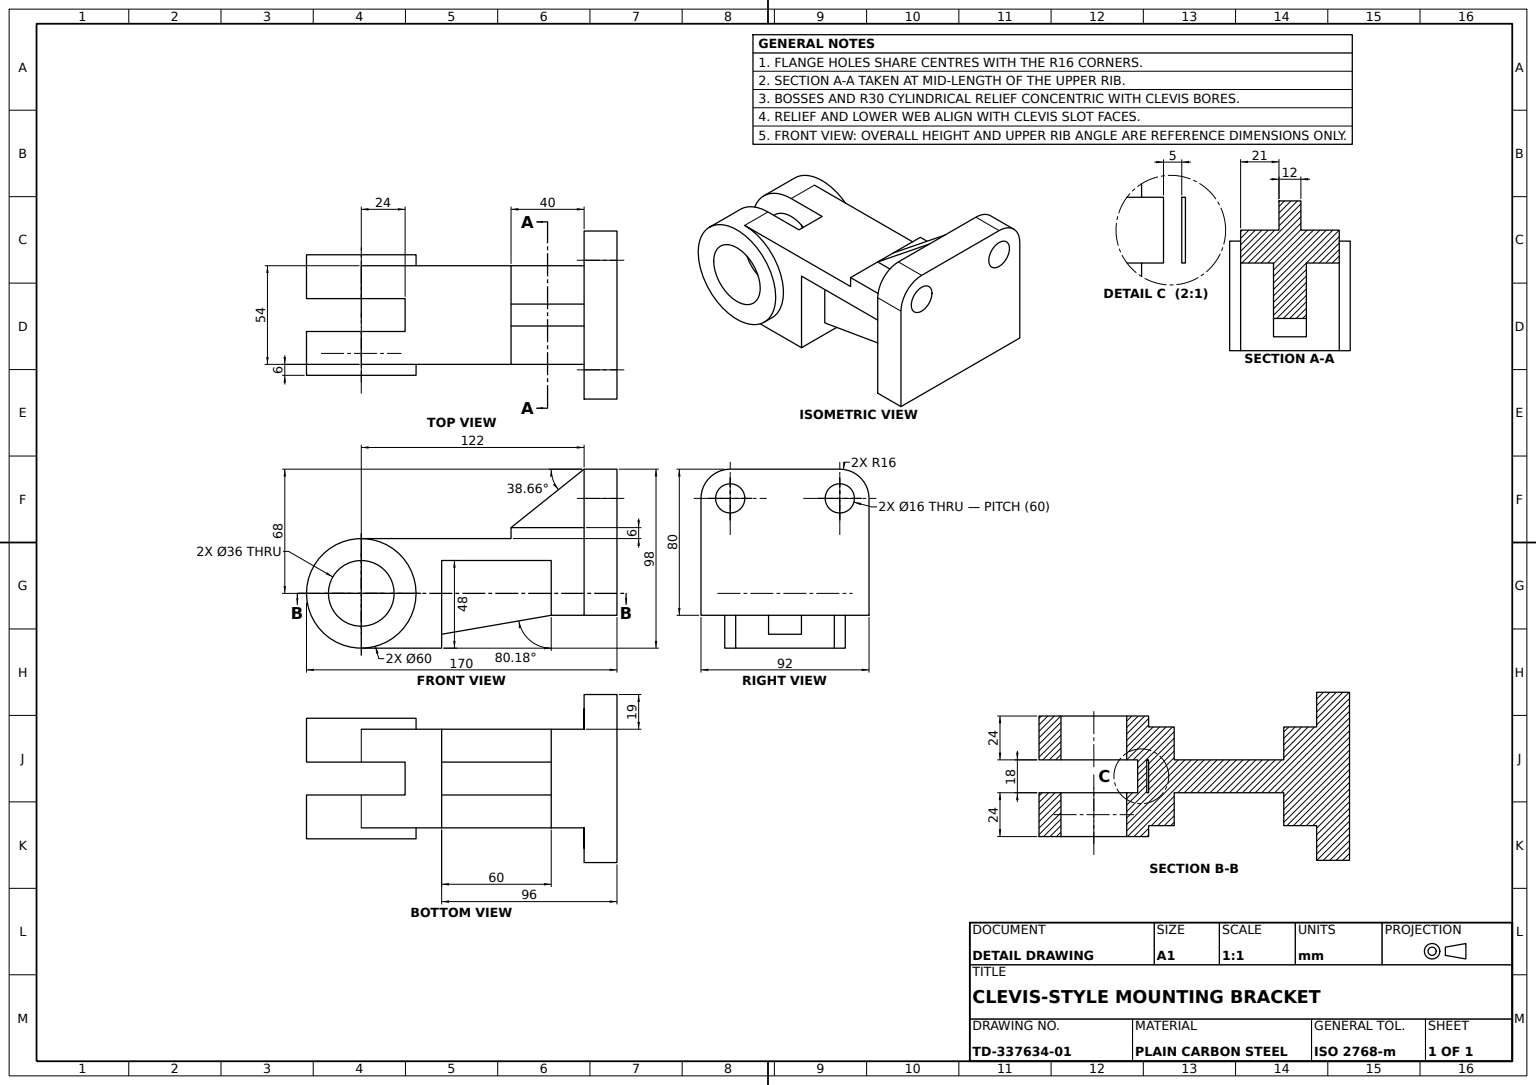
from build123d import *

# Parameters (mm, degrees)
HUB_PROFILE_SKETCH_R         = 30
HUB_60_DEPTH                 = 24
HUB_EXTENSION_SKETCH_R       = 30
HUB_EXTENSION_60_DEPTH       = 24
HUB_BORE_SKETCH_R            = 18
HUB_BORE_36_DEPTH            = 98
ARM_START                    = -54
ARM_BODY_DEPTH               = 54
CLEVIS_SLOT_SKETCH_W         = 24
CLEVIS_SLOT_SKETCH_H         = 18
CLEVIS_SLOT_24MM_DEPTH       = 96
SLOT_PAD_SKETCH_W            = 18
SLOT_PAD_SKETCH_H            = 60
SLOT_PAD_5MM_DEPTH           = 5
RIB_BASE_PAD_SKETCH_W        = 40
RIB_BASE_PAD_SKETCH_H        = 54
RIB_BASE_PAD_DEPTH           = 6
MOUNTING_FLANGE_SKETCH_W     = 18
MOUNTING_FLANGE_SKETCH_H     = 80
MOUNTING_FLANGE_DEPTH        = 46
FLANGE_CORNER_FILLET_R16_A_R = 16
FLANGE_CORNER_FILLET_R16_B_R = 16
FLANGE_HOLES_SKETCH_R        = 8
FLANGE_HOLES_2X_16_DEPTH     = 92
FLANGE_RIB_12MM_REACH        = 164.296
FLANGE_RIB_SKETCH_WALL_W     = 377.817045558
FLANGE_RIB_SKETCH_WALL_H     = 12
ARM_RELIEF_CUT_DEPTH         = 92
ARM_RIB_18MM_REACH           = 164.296
ARM_RIB_SKETCH_WALL_W        = 432.138250074
ARM_RIB_SKETCH_WALL_H        = 18


with BuildPart() as part:
    # Hub Profile Sketch → Hub Ø60 (new body)
    with BuildSketch(Plane.XY):
        Circle(HUB_PROFILE_SKETCH_R)
    extrude(amount=HUB_60_DEPTH)


with BuildPart() as body_2:
    # Hub Extension Sketch → Hub Extension Ø60 (new body)
    with BuildSketch(Plane(origin=(0, 0, -18), x_dir=(-1, 0, 0), z_dir=(0, 0, -1))):
        with Locations(Location((0, 0, 0), (0, 0, 180))):
            Circle(HUB_EXTENSION_SKETCH_R)
    extrude(amount=HUB_EXTENSION_60_DEPTH)


with BuildPart() as hub_bore_36_tool:
    # Hub Bore Sketch → Hub Bore Ø36 (new body)
    with BuildSketch(Plane.XY.offset(24)):
        Circle(HUB_BORE_SKETCH_R)
    extrude(amount=-HUB_BORE_36_DEPTH)


with BuildPart() as part_1:
    add(part.part)

    # Hub Bore Ø36: cut by hub_bore_36_tool
    add(hub_bore_36_tool.part, mode=Mode.SUBTRACT)



with BuildPart() as body_2_1:
    add(body_2.part)

    # Hub Bore Ø36: cut by hub_bore_36_tool
    add(hub_bore_36_tool.part, mode=Mode.SUBTRACT)


with BuildPart() as part_2:
    add(part_1.part)

    add(body_2_1.part)  # Arm Body merges body 2
    # Arm Profile Sketch → Arm Body (add)
    with BuildSketch(Plane.XY.offset(18).offset(ARM_START)):
        with BuildLine():
            Line((0, 30), (122, 30))
            Line((122, 30), (122, -30))
            Line((122, -30), (0, -30))
            ThreePointArc((0, -30), (30, 0), (0, 30))
        make_face()
    extrude(amount=ARM_BODY_DEPTH)

    # Clevis Slot Sketch → Clevis Slot 24mm (cut)
    with BuildSketch(Plane(origin=(0, 30, 0), x_dir=(1, 0, 0), z_dir=(0, 1, 0))):
        with Locations((12, 9)):
            Rectangle(CLEVIS_SLOT_SKETCH_W, CLEVIS_SLOT_SKETCH_H)
    extrude(amount=-CLEVIS_SLOT_24MM_DEPTH, mode=Mode.SUBTRACT)

    # Slot Pad Sketch → Slot Pad 5mm (add)
    with BuildSketch(Plane.ZY.offset(-24)):
        with Locations((-9, 0)):
            Rectangle(SLOT_PAD_SKETCH_W, SLOT_PAD_SKETCH_H)
    extrude(amount=-SLOT_PAD_5MM_DEPTH)

    # Rib Base Pad Sketch → Rib Base Pad (add)
    with BuildSketch(Plane(origin=(0, 30, 0), x_dir=(1, 0, 0), z_dir=(0, 1, 0))):
        with Locations((102, 9)):
            Rectangle(RIB_BASE_PAD_SKETCH_W, RIB_BASE_PAD_SKETCH_H)
    extrude(amount=RIB_BASE_PAD_DEPTH)

    # Mounting Flange Sketch → Mounting Flange (add, symmetric)
    with BuildSketch(Plane(origin=(0, 0, -9), x_dir=(-1, 0, 0), z_dir=(0, 0, -1))):
        with Locations((-131, 28)):
            Rectangle(MOUNTING_FLANGE_SKETCH_W, MOUNTING_FLANGE_SKETCH_H)
    extrude(amount=MOUNTING_FLANGE_DEPTH, both=True)

    # Flange Corner Fillet R16 A
    flange_corner_fillet_r16_a_edges = [part_2.edges().sort_by_distance(p)[0] for p in [
        (131, 68, 37),
    ]]
    fillet(flange_corner_fillet_r16_a_edges, radius=FLANGE_CORNER_FILLET_R16_A_R)

    # Flange Corner Fillet R16 B
    flange_corner_fillet_r16_b_edges = [part_2.edges().sort_by_distance(p)[0] for p in [
        (131, 68, -55),
    ]]
    fillet(flange_corner_fillet_r16_b_edges, radius=FLANGE_CORNER_FILLET_R16_B_R)

    # Flange Holes Sketch → Flange Holes 2xØ16 (cut)
    with BuildSketch(Plane.ZY.offset(-122)):
        with Locations((21, 52)):
            Circle(FLANGE_HOLES_SKETCH_R)
        with Locations((-39, 52)):
            Circle(FLANGE_HOLES_SKETCH_R)
    extrude(amount=-FLANGE_HOLES_2X_16_DEPTH, mode=Mode.SUBTRACT)

    # Flange Rib Sketch wall → Flange Rib 12mm (add, up to next)
    with BuildSketch(Plane(origin=(102, 52, -9), x_dir=(0.780868809443, 0.624695047554, 0), z_dir=(0.624695047554, -0.780868809443, 0)), mode=Mode.PRIVATE) as flange_rib_12mm_sk1:
        Rectangle(FLANGE_RIB_SKETCH_WALL_W, FLANGE_RIB_SKETCH_WALL_H)
    flange_rib_12mm_tool1 = extrude(flange_rib_12mm_sk1.sketch, amount=FLANGE_RIB_12MM_REACH, mode=Mode.PRIVATE) - part_2.part
    add(flange_rib_12mm_tool1.solids().sort_by_distance((102, 52, -9))[0])

    # Arm Relief Sketch → Arm Relief Cut (cut)
    with BuildSketch(Plane.XY.offset(18)):
        Polygon((104, 18), (104, -12), (44, -30), (44, 18), align=None)
        Polygon((122, -30), (122, -12), (104, -12), (44, -30), align=None)
    extrude(amount=-ARM_RELIEF_CUT_DEPTH, mode=Mode.SUBTRACT)

    # Arm Rib Sketch wall → Arm Rib 18mm (add, up to next)
    with BuildSketch(Plane(origin=(52, -21, -9), x_dir=(0.985350505855, 0.170541433706, 0), z_dir=(0.170541433706, -0.985350505855, 0)), mode=Mode.PRIVATE) as arm_rib_18mm_sk1:
        Rectangle(ARM_RIB_SKETCH_WALL_W, ARM_RIB_SKETCH_WALL_H)
    arm_rib_18mm_tool1 = extrude(arm_rib_18mm_sk1.sketch, amount=-ARM_RIB_18MM_REACH, mode=Mode.PRIVATE) - part_2.part
    add(arm_rib_18mm_tool1.solids().sort_by_distance((52, -21, -9))[0])


solid = part_2.part
